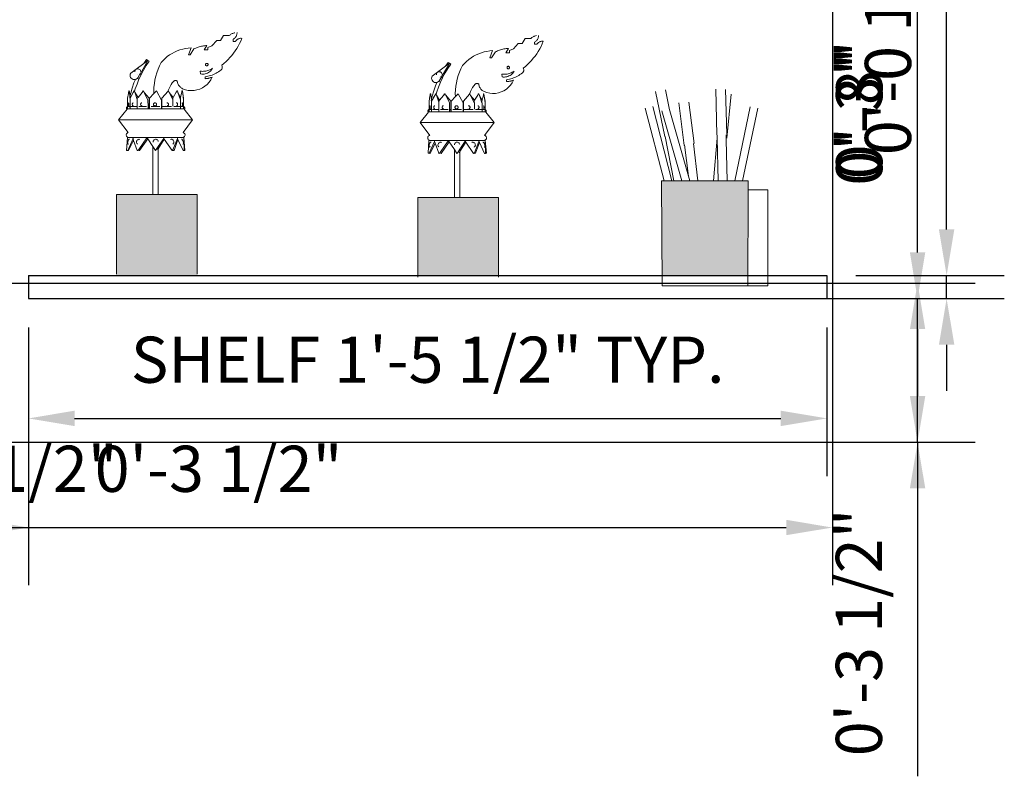
# Model space of a CAD drawing. Units: millimetres. Extents: x 7894 to 8038, y 6851 to 6951.
# Tile 7 of 49: x 7963.22 to 7984.56, y 6854.37 to 6870.77. Entities that reach past the tile are written whole.
import ezdxf

# ---------------------------------------------------------------- set-up
doc = ezdxf.new("R2010")
doc.units = ezdxf.units.MM
for name, color, linetype, lineweight in [('A-ANNO-DIMS', 2, 'Continuous', 18), ('A-FURN-ACCS', 8, 'Continuous', 13), ('A-FURN-SHLF', 7, 'Continuous', 30)]:
    doc.layers.add(name, color=color, linetype=linetype, lineweight=lineweight)
doc.layers.add('A-FURN-ACCS-PATT', color=116, linetype='Continuous', lineweight=9, true_color=0x136734)
doc.styles.get("Standard").update_dxf_attribs({"font": 'arial.ttf'})
doc.dimstyles.new('ISO-25', dxfattribs={"dimtxt": 1, "dimasz": 1, "dimexe": 1.25, "dimexo": 0.625, "dimtad": 1, "dimdec": 0, "dimlunit": 4, "dimtxsty": 'Standard', "dimcen": 2.5, "dimclrt": 1, "dimadec": 0, "dimazin": 0, "dimtfac": 1, "dimtdec": 0, "dimtmove": 0, "dimatfit": 3, "dimfxl": 1, "dimarcsym": 0})

# ---------------------------------------------------------------- blocks, each defined once
blk = doc.blocks.new('FLOATING-SHELF-ELEV')
for p, q in [((0, 0.5), (17.304, 0.5)), ((0, 0.5), (0, 0)), ((17.304, 0.5), (17.304, 0)), ((0, 0), (17.304, 0))]:
    blk.add_line(p, q)
blk = doc.blocks.new('DISPLAY-LEAF-FINIAL')
for p, q in [((2.209, 3.334), (2.276, 3.441)), ((2.276, 3.441), (2.398, 3.441)), ((2.398, 3.441), (2.409, 3.452)), ((2.409, 3.452), (2.421, 3.461)), ((2.421, 3.461), (2.434, 3.47)), ((2.434, 3.47), (2.447, 3.478)), ((2.447, 3.478), (2.461, 3.485)), ((2.461, 3.485), (2.475, 3.491)), ((2.475, 3.491), (2.489, 3.496)), ((2.489, 3.496), (2.504, 3.501)), ((2.504, 3.501), (2.519, 3.504)), ((2.544, 3.424), (2.536, 3.411)), ((2.551, 3.437), (2.544, 3.424)), ((2.556, 3.45), (2.551, 3.437)), ((2.56, 3.465), (2.556, 3.45)), ((2.563, 3.479), (2.56, 3.465)), ((2.565, 3.494), (2.563, 3.479)), ((2.565, 3.508), (2.565, 3.494)), ((1.745, 3.198), (1.769, 3.205)), ((1.769, 3.205), (1.793, 3.211)), ((1.793, 3.211), (1.817, 3.216)), ((1.817, 3.216), (1.841, 3.22)), ((1.841, 3.22), (1.865, 3.223)), ((1.914, 3.227), (1.854, 3.133)), ((1.865, 3.223), (1.889, 3.226)), ((1.889, 3.226), (1.914, 3.227)), ((1.934, 3.185), (2.023, 3.221)), ((2.023, 3.221), (2.127, 3.334)), ((2.127, 3.334), (2.209, 3.334)), ((2.493, 3.371), (2.48, 3.364)), ((2.48, 3.364), (2.48, 3.316)), ((2.48, 3.316), (2.533, 3.316)), ((2.505, 3.379), (2.493, 3.371)), ((2.516, 3.389), (2.505, 3.379)), ((2.527, 3.4), (2.516, 3.389)), ((2.536, 3.411), (2.527, 3.4)), ((2.533, 3.316), (2.54, 3.327)), ((2.54, 3.327), (2.549, 3.338)), ((2.549, 3.338), (2.558, 3.347)), ((2.558, 3.347), (2.569, 3.356)), ((2.591, 3.216), (2.56, 3.163)), ((2.569, 3.356), (2.58, 3.363)), ((2.58, 3.363), (2.592, 3.37)), ((2.62, 3.27), (2.591, 3.216)), ((2.592, 3.37), (2.604, 3.375)), ((2.604, 3.375), (2.617, 3.379)), ((2.617, 3.379), (2.63, 3.382)), ((2.646, 3.325), (2.62, 3.27)), ((2.63, 3.382), (2.643, 3.383)), ((2.643, 3.383), (2.657, 3.383)), ((2.67, 3.382), (2.646, 3.325)), ((2.657, 3.383), (2.67, 3.382)), ((1.055, 2.986), (1.105, 3.023)), ((1.105, 3.023), (1.158, 3.056)), ((1.158, 3.056), (1.213, 3.085)), ((1.213, 3.085), (1.27, 3.111)), ((1.27, 3.111), (1.328, 3.133)), ((1.328, 3.133), (1.388, 3.15)), ((1.388, 3.15), (1.449, 3.164)), ((1.449, 3.164), (1.51, 3.173)), ((1.51, 3.173), (1.572, 3.179)), ((1.572, 3.179), (1.511, 3.024)), ((1.511, 3.024), (1.55, 3.024)), ((1.55, 3.024), (1.632, 3.152)), ((1.632, 3.152), (1.654, 3.163)), ((1.654, 3.163), (1.676, 3.173)), ((1.676, 3.173), (1.699, 3.182)), ((1.699, 3.182), (1.722, 3.191)), ((1.722, 3.191), (1.745, 3.198)), ((1.854, 3.133), (1.934, 3.133)), ((1.934, 3.133), (1.934, 3.185)), ((2.453, 3.014), (2.413, 2.967)), ((2.491, 3.062), (2.453, 3.014)), ((2.527, 3.112), (2.491, 3.062)), ((2.56, 3.163), (2.527, 3.112)), ((0.547, 2.84), (0.379, 2.713)), ((0.634, 2.9), (0.463, 2.609)), ((0.541, 2.696), (0.599, 2.791)), ((0.605, 2.924), (0.547, 2.84)), ((0.634, 2.905), (0.547, 2.84)), ((0.599, 2.791), (0.663, 2.885)), ((0.634, 2.905), (0.605, 2.924)), ((0.634, 2.9), (0.634, 2.905)), ((0.663, 2.885), (0.634, 2.905)), ((0.884, 2.786), (0.853, 2.713)), ((0.92, 2.857), (0.884, 2.786)), ((0.92, 2.857), (0.962, 2.903)), ((0.962, 2.903), (1.007, 2.946)), ((1.007, 2.946), (1.055, 2.986)), ((1.883, 2.817), (1.885, 2.824)), ((1.883, 2.81), (1.883, 2.817)), ((1.885, 2.803), (1.883, 2.81)), ((1.885, 2.824), (1.889, 2.831)), ((1.888, 2.797), (1.885, 2.803)), ((1.894, 2.791), (1.888, 2.797)), ((1.889, 2.831), (1.894, 2.836)), ((1.894, 2.836), (1.9, 2.839)), ((1.9, 2.788), (1.894, 2.791)), ((1.9, 2.839), (1.907, 2.841)), ((1.907, 2.786), (1.9, 2.788)), ((1.907, 2.841), (1.914, 2.841)), ((1.914, 2.786), (1.907, 2.786)), ((1.914, 2.841), (1.921, 2.839)), ((1.921, 2.788), (1.914, 2.786)), ((1.921, 2.839), (1.928, 2.836)), ((1.928, 2.791), (1.921, 2.788)), ((1.928, 2.836), (1.933, 2.83)), ((1.933, 2.796), (1.928, 2.791)), ((1.933, 2.83), (1.937, 2.824)), ((1.936, 2.803), (1.933, 2.796)), ((1.938, 2.81), (1.936, 2.803)), ((1.937, 2.824), (1.938, 2.817)), ((1.938, 2.817), (1.938, 2.81)), ((2.281, 2.839), (2.233, 2.801)), ((2.233, 2.801), (2.238, 2.792)), ((2.238, 2.792), (2.242, 2.783)), ((2.242, 2.783), (2.245, 2.774)), ((2.327, 2.88), (2.281, 2.839)), ((2.371, 2.923), (2.327, 2.88)), ((2.413, 2.967), (2.371, 2.923)), ((0.253, 2.607), (0.249, 2.584)), ((0.249, 2.58), (0.249, 2.584)), ((0.249, 2.58), (0.251, 2.557)), ((0.264, 2.627), (0.253, 2.607)), ((0.379, 2.713), (0.264, 2.627)), ((0.353, 2.675), (0.358, 2.69)), ((0.353, 2.66), (0.353, 2.675)), ((0.353, 2.659), (0.353, 2.66)), ((0.353, 2.657), (0.353, 2.659)), ((0.358, 2.69), (0.367, 2.703)), ((0.367, 2.703), (0.379, 2.713)), ((0.379, 2.713), (0.393, 2.72)), ((0.393, 2.72), (0.409, 2.723)), ((0.409, 2.723), (0.425, 2.722)), ((0.414, 2.606), (0.413, 2.603)), ((0.461, 2.605), (0.415, 2.527)), ((0.425, 2.722), (0.44, 2.718)), ((0.44, 2.718), (0.453, 2.709)), ((0.44, 2.496), (0.486, 2.593)), ((0.443, 2.613), (0.446, 2.612)), ((0.451, 2.615), (0.449, 2.616)), ((0.453, 2.709), (0.464, 2.698)), ((0.463, 2.609), (0.461, 2.605)), ((0.486, 2.593), (0.461, 2.605)), ((0.463, 2.609), (0.488, 2.597)), ((0.464, 2.698), (0.471, 2.684)), ((0.471, 2.684), (0.475, 2.669)), ((0.474, 2.667), (0.475, 2.669)), ((0.474, 2.667), (0.475, 2.666)), ((0.541, 2.696), (0.488, 2.597)), ((0.804, 2.562), (0.787, 2.485)), ((0.826, 2.638), (0.804, 2.562)), ((0.853, 2.713), (0.826, 2.638)), ((1.793, 2.668), (1.77, 2.67)), ((1.77, 2.67), (1.776, 2.611)), ((1.801, 2.608), (1.776, 2.611)), ((1.816, 2.667), (1.793, 2.668)), ((1.827, 2.607), (1.801, 2.608)), ((1.84, 2.668), (1.816, 2.667)), ((1.852, 2.609), (1.827, 2.607)), ((1.863, 2.67), (1.84, 2.668)), ((1.878, 2.613), (1.852, 2.609)), ((1.886, 2.673), (1.863, 2.67)), ((1.902, 2.62), (1.878, 2.613)), ((1.909, 2.678), (1.886, 2.673)), ((1.926, 2.63), (1.902, 2.62)), ((1.931, 2.684), (1.909, 2.678)), ((1.949, 2.642), (1.926, 2.63)), ((1.954, 2.692), (1.931, 2.684)), ((1.964, 2.569), (1.934, 2.561)), ((1.97, 2.657), (1.949, 2.642)), ((1.975, 2.701), (1.954, 2.692)), ((1.994, 2.578), (1.964, 2.569)), ((1.99, 2.673), (1.97, 2.657)), ((1.996, 2.711), (1.975, 2.701)), ((2.007, 2.692), (1.99, 2.673)), ((2.024, 2.588), (1.994, 2.578)), ((2.017, 2.722), (1.996, 2.711)), ((2.023, 2.712), (2.007, 2.692)), ((2.036, 2.734), (2.017, 2.722)), ((2.036, 2.734), (2.023, 2.712)), ((2.053, 2.6), (2.024, 2.588)), ((2.082, 2.613), (2.053, 2.6)), ((2.11, 2.627), (2.082, 2.613)), ((2.137, 2.643), (2.11, 2.627)), ((2.164, 2.659), (2.137, 2.643)), ((2.19, 2.677), (2.164, 2.659)), ((2.216, 2.695), (2.19, 2.677)), ((2.223, 2.702), (2.216, 2.695)), ((2.23, 2.709), (2.223, 2.702)), ((2.235, 2.717), (2.23, 2.709)), ((2.24, 2.726), (2.235, 2.717)), ((2.243, 2.735), (2.24, 2.726)), ((2.245, 2.745), (2.243, 2.735)), ((2.245, 2.774), (2.246, 2.764)), ((2.246, 2.754), (2.245, 2.745)), ((2.246, 2.764), (2.246, 2.754)), ((0.251, 2.557), (0.259, 2.536)), ((0.259, 2.536), (0.272, 2.517)), ((0.272, 2.517), (0.29, 2.502)), ((0.29, 2.502), (0.311, 2.492)), ((0.332, 2.415), (0.295, 2.306)), ((0.311, 2.492), (0.334, 2.488)), ((0.363, 2.491), (0.332, 2.415)), ((0.334, 2.488), (0.358, 2.489)), ((0.358, 2.489), (0.363, 2.491)), ((0.361, 2.285), (0.398, 2.391)), ((0.363, 2.491), (0.38, 2.497)), ((0.365, 2.496), (0.363, 2.491)), ((0.38, 2.497), (0.4, 2.51)), ((0.398, 2.513), (0.402, 2.512)), ((0.398, 2.391), (0.44, 2.495)), ((0.403, 2.513), (0.4, 2.514)), ((0.4, 2.51), (0.402, 2.512)), ((0.402, 2.512), (0.403, 2.513)), ((0.402, 2.512), (0.44, 2.495)), ((0.403, 2.513), (0.415, 2.527)), ((0.403, 2.513), (0.44, 2.496)), ((0.409, 2.511), (0.408, 2.509)), ((0.42, 2.535), (0.409, 2.511)), ((0.774, 2.406), (0.766, 2.327)), ((0.787, 2.485), (0.774, 2.406)), ((1.136, 2.379), (1.113, 2.339)), ((1.163, 2.417), (1.136, 2.379)), ((1.193, 2.452), (1.163, 2.417)), ((1.198, 2.457), (1.193, 2.452)), ((1.204, 2.462), (1.198, 2.457)), ((1.211, 2.465), (1.204, 2.462)), ((1.218, 2.467), (1.211, 2.465)), ((1.225, 2.469), (1.218, 2.467)), ((1.232, 2.47), (1.225, 2.469)), ((1.239, 2.469), (1.232, 2.47)), ((1.247, 2.467), (1.239, 2.469)), ((1.254, 2.465), (1.247, 2.467)), ((1.26, 2.462), (1.254, 2.465)), ((1.266, 2.457), (1.26, 2.462)), ((1.271, 2.452), (1.266, 2.457)), ((1.274, 2.435), (1.271, 2.452)), ((1.278, 2.418), (1.274, 2.435)), ((1.283, 2.402), (1.278, 2.418)), ((1.29, 2.386), (1.283, 2.402)), ((1.298, 2.371), (1.29, 2.386)), ((1.308, 2.357), (1.298, 2.371)), ((1.319, 2.343), (1.308, 2.357)), ((1.918, 2.385), (1.87, 2.344)), ((1.903, 2.554), (1.872, 2.548)), ((1.872, 2.548), (1.872, 2.508)), ((1.872, 2.508), (1.885, 2.509)), ((1.885, 2.509), (1.898, 2.51)), ((1.898, 2.51), (1.911, 2.511)), ((1.934, 2.561), (1.903, 2.554)), ((1.911, 2.511), (1.924, 2.513)), ((1.961, 2.432), (1.918, 2.385)), ((1.924, 2.513), (1.937, 2.515)), ((1.937, 2.515), (1.95, 2.518)), ((1.95, 2.518), (1.963, 2.521)), ((1.997, 2.484), (1.961, 2.432)), ((1.963, 2.521), (1.976, 2.524)), ((1.976, 2.524), (1.988, 2.528)), ((1.988, 2.528), (2.001, 2.532)), ((2.026, 2.541), (1.997, 2.484)), ((2.001, 2.532), (2.013, 2.536)), ((2.013, 2.536), (2.026, 2.541)), ((0.213, 2.19), (0.195, 2.086)), ((0.213, 2.19), (0.215, 2.201)), ((0.215, 2.201), (0.22, 2.245)), ((0.223, 2.245), (0.215, 2.201)), ((0.223, 2.245), (0.22, 2.245)), ((0.223, 2.245), (0.23, 2.245)), ((0.232, 2.22), (0.23, 2.245)), ((0.232, 2.22), (0.25, 2.138)), ((0.244, 2.11), (0.232, 2.22)), ((0.25, 2.138), (0.244, 2.11)), ((0.317, 2.207), (0.248, 2.086)), ((0.263, 2.194), (0.25, 2.138)), ((0.25, 2.138), (0.256, 2.115)), ((0.295, 2.306), (0.263, 2.194)), ((0.297, 2.185), (0.292, 2.162)), ((0.317, 2.207), (0.33, 2.245)), ((0.338, 2.245), (0.317, 2.207)), ((0.332, 2.245), (0.33, 2.245)), ((0.344, 2.245), (0.338, 2.245)), ((0.347, 2.235), (0.344, 2.245)), ((0.347, 2.235), (0.361, 2.285)), ((0.354, 2.213), (0.347, 2.235)), ((0.354, 2.213), (0.42, 2.104)), ((0.404, 2.061), (0.354, 2.213)), ((0.507, 2.209), (0.42, 2.104)), ((0.507, 2.209), (0.525, 2.245)), ((0.532, 2.239), (0.507, 2.209)), ((0.528, 2.245), (0.525, 2.245)), ((0.528, 2.245), (0.532, 2.239)), ((0.537, 2.245), (0.532, 2.239)), ((0.54, 2.245), (0.537, 2.245)), ((0.556, 2.211), (0.54, 2.245)), ((0.548, 2.22), (0.556, 2.211)), ((0.556, 2.211), (0.663, 2.086)), ((0.636, 2.045), (0.556, 2.211)), ((0.765, 2.186), (0.671, 2.086)), ((0.766, 2.327), (0.763, 2.248)), ((0.763, 2.248), (0.765, 2.186)), ((0.821, 2.245), (0.765, 2.186)), ((0.93, 2.045), (0.821, 2.245)), ((1.07, 2.239), (0.939, 2.086)), ((1.07, 2.239), (1.069, 2.235)), ((1.071, 2.24), (1.07, 2.239)), ((1.07, 2.239), (1.071, 2.237)), ((1.075, 2.254), (1.071, 2.24)), ((1.074, 2.245), (1.071, 2.24)), ((1.074, 2.245), (1.078, 2.245)), ((1.092, 2.297), (1.075, 2.254)), ((1.095, 2.209), (1.078, 2.245)), ((1.113, 2.339), (1.092, 2.297)), ((1.095, 2.209), (1.182, 2.104)), ((1.095, 2.209), (1.171, 2.054)), ((1.248, 2.213), (1.182, 2.104)), ((1.248, 2.213), (1.258, 2.245)), ((1.265, 2.242), (1.248, 2.213)), ((1.258, 2.245), (1.264, 2.245)), ((1.264, 2.245), (1.265, 2.242)), ((1.267, 2.245), (1.265, 2.242)), ((1.267, 2.245), (1.272, 2.245)), ((1.285, 2.207), (1.272, 2.245)), ((1.285, 2.207), (1.344, 2.103)), ((1.285, 2.207), (1.34, 2.048)), ((1.331, 2.331), (1.319, 2.343)), ((1.343, 2.319), (1.331, 2.331)), ((1.357, 2.309), (1.343, 2.319)), ((1.37, 2.22), (1.344, 2.103)), ((1.372, 2.3), (1.357, 2.309)), ((1.37, 2.22), (1.372, 2.245)), ((1.375, 2.245), (1.37, 2.22)), ((1.387, 2.292), (1.372, 2.3)), ((1.372, 2.245), (1.375, 2.245)), ((1.375, 2.245), (1.382, 2.245)), ((1.382, 2.245), (1.389, 2.19)), ((1.447, 2.27), (1.387, 2.292)), ((1.389, 2.19), (1.408, 2.086)), ((1.407, 2.045), (1.389, 2.19)), ((1.509, 2.256), (1.447, 2.27)), ((1.572, 2.25), (1.509, 2.256)), ((1.635, 2.253), (1.572, 2.25)), ((1.698, 2.264), (1.635, 2.253)), ((1.759, 2.283), (1.698, 2.264)), ((1.816, 2.31), (1.759, 2.283)), ((1.87, 2.344), (1.816, 2.31)), ((0.195, 2.086), (0.195, 2.048)), ((0.195, 2.045), (0.195, 2.048)), ((0.195, 2.045), (0.195, 1.903)), ((0.207, 1.965), (0.208, 1.973)), ((0.207, 1.956), (0.207, 1.965)), ((0.207, 1.947), (0.207, 1.956)), ((0.207, 1.938), (0.207, 1.947)), ((0.208, 1.93), (0.207, 1.938)), ((0.208, 1.973), (0.209, 1.979)), ((0.209, 1.924), (0.208, 1.93)), ((0.209, 1.979), (0.211, 1.984)), ((0.211, 1.919), (0.209, 1.924)), ((0.21, 1.956), (0.211, 1.965)), ((0.21, 1.947), (0.21, 1.956)), ((0.211, 1.938), (0.21, 1.947)), ((0.211, 1.984), (0.213, 1.986)), ((0.211, 1.965), (0.212, 1.973)), ((0.212, 1.93), (0.211, 1.938)), ((0.212, 1.973), (0.213, 1.979)), ((0.213, 1.924), (0.212, 1.93)), ((0.216, 1.986), (0.213, 1.986)), ((0.213, 1.979), (0.214, 1.984)), ((0.216, 1.947), (0.213, 1.924)), ((0.214, 1.919), (0.213, 1.924)), ((0.214, 1.984), (0.216, 1.986)), ((0.217, 1.965), (0.216, 1.956)), ((0.216, 1.956), (0.216, 1.947)), ((0.216, 1.947), (0.217, 1.938)), ((0.218, 1.973), (0.217, 1.965)), ((0.218, 1.967), (0.217, 1.965)), ((0.217, 1.938), (0.218, 1.93)), ((0.219, 1.979), (0.218, 1.973)), ((0.218, 1.973), (0.218, 1.967)), ((0.218, 1.93), (0.219, 1.924)), ((0.22, 1.981), (0.219, 1.979)), ((0.22, 1.981), (0.219, 1.979)), ((0.219, 1.924), (0.22, 1.921)), ((0.221, 1.973), (0.22, 1.965)), ((0.22, 1.965), (0.22, 1.956)), ((0.22, 1.956), (0.22, 1.947)), ((0.22, 1.947), (0.22, 1.938)), ((0.22, 1.938), (0.221, 1.93)), ((0.222, 1.975), (0.221, 1.973)), ((0.221, 1.93), (0.222, 1.928)), ((0.244, 2.11), (0.239, 2.089)), ((0.248, 2.065), (0.244, 2.11)), ((0.248, 1.925), (0.246, 1.901)), ((0.248, 2.086), (0.248, 2.065)), ((0.248, 2.065), (0.248, 1.903)), ((0.295, 1.956), (0.297, 1.965)), ((0.295, 1.947), (0.295, 1.956)), ((0.297, 1.938), (0.295, 1.947)), ((0.297, 1.965), (0.3, 1.973)), ((0.3, 1.93), (0.297, 1.938)), ((0.3, 1.973), (0.304, 1.979)), ((0.303, 1.924), (0.3, 1.93)), ((0.308, 1.919), (0.303, 1.924)), ((0.304, 1.979), (0.308, 1.984)), ((0.308, 1.984), (0.314, 1.986)), ((0.316, 1.986), (0.314, 1.986)), ((0.42, 2.104), (0.404, 2.086)), ((0.404, 2.086), (0.404, 2.061)), ((0.404, 2.061), (0.404, 1.901)), ((0.476, 1.956), (0.478, 1.965)), ((0.476, 1.947), (0.476, 1.956)), ((0.478, 1.938), (0.476, 1.947)), ((0.478, 1.965), (0.482, 1.973)), ((0.482, 1.93), (0.478, 1.938)), ((0.482, 1.973), (0.488, 1.979)), ((0.488, 1.924), (0.482, 1.93)), ((0.488, 1.979), (0.495, 1.984)), ((0.495, 1.919), (0.488, 1.924)), ((0.495, 1.984), (0.502, 1.986)), ((0.504, 1.986), (0.502, 1.986)), ((0.636, 2.045), (0.637, 1.903)), ((0.663, 2.086), (0.663, 1.903)), ((0.671, 2.086), (0.671, 1.903)), ((0.754, 1.956), (0.756, 1.965)), ((0.754, 1.947), (0.754, 1.956)), ((0.756, 1.938), (0.754, 1.947)), ((0.756, 1.965), (0.761, 1.973)), ((0.761, 1.93), (0.756, 1.938)), ((0.761, 1.973), (0.767, 1.979)), ((0.767, 1.924), (0.761, 1.93)), ((0.767, 1.979), (0.775, 1.984)), ((0.775, 1.919), (0.767, 1.924)), ((0.775, 1.984), (0.784, 1.986)), ((0.784, 1.986), (0.793, 1.986)), ((0.793, 1.986), (0.802, 1.984)), ((0.802, 1.984), (0.81, 1.979)), ((0.81, 1.924), (0.802, 1.919)), ((0.81, 1.979), (0.816, 1.973)), ((0.816, 1.93), (0.81, 1.924)), ((0.816, 1.973), (0.821, 1.965)), ((0.821, 1.938), (0.816, 1.93)), ((0.821, 1.965), (0.823, 1.956)), ((0.823, 1.947), (0.821, 1.938)), ((0.823, 1.956), (0.823, 1.947)), ((0.93, 2.045), (0.931, 1.934)), ((0.939, 1.934), (0.931, 1.934)), ((0.931, 1.934), (0.931, 1.903)), ((0.939, 2.086), (0.939, 1.934)), ((0.942, 1.934), (0.939, 1.934)), ((0.939, 1.934), (0.939, 1.903)), ((1.022, 1.935), (1.021, 1.935)), ((1.044, 1.986), (1.046, 1.986)), ((1.046, 1.986), (1.054, 1.986)), ((1.054, 1.986), (1.062, 1.984)), ((1.062, 1.984), (1.069, 1.979)), ((1.069, 1.924), (1.062, 1.919)), ((1.069, 1.979), (1.075, 1.973)), ((1.075, 1.93), (1.069, 1.924)), ((1.075, 1.973), (1.079, 1.965)), ((1.079, 1.938), (1.075, 1.93)), ((1.079, 1.965), (1.081, 1.956)), ((1.081, 1.947), (1.079, 1.938)), ((1.081, 1.956), (1.081, 1.947)), ((1.182, 2.104), (1.171, 2.086)), ((1.171, 2.086), (1.171, 2.054)), ((1.176, 2.045), (1.171, 2.054)), ((1.176, 2.045), (1.177, 1.914)), ((1.249, 1.986), (1.251, 1.986)), ((1.251, 1.986), (1.257, 1.986)), ((1.257, 1.986), (1.263, 1.984)), ((1.263, 1.984), (1.268, 1.979)), ((1.268, 1.924), (1.263, 1.919)), ((1.268, 1.979), (1.272, 1.973)), ((1.272, 1.93), (1.268, 1.924)), ((1.272, 1.973), (1.275, 1.965)), ((1.275, 1.938), (1.272, 1.93)), ((1.275, 1.965), (1.276, 1.956)), ((1.276, 1.947), (1.275, 1.938)), ((1.276, 1.956), (1.276, 1.947)), ((1.344, 2.103), (1.34, 2.086)), ((1.34, 2.086), (1.34, 2.048)), ((1.341, 2.045), (1.34, 2.048)), ((1.341, 2.045), (1.342, 1.903)), ((1.373, 1.986), (1.376, 1.986)), ((1.376, 1.986), (1.378, 1.984)), ((1.376, 1.986), (1.377, 1.986)), ((1.377, 1.986), (1.379, 1.986)), ((1.378, 1.984), (1.379, 1.979)), ((1.379, 1.924), (1.378, 1.919)), ((1.379, 1.986), (1.381, 1.984)), ((1.379, 1.979), (1.381, 1.973)), ((1.381, 1.93), (1.379, 1.924)), ((1.381, 1.984), (1.383, 1.979)), ((1.381, 1.973), (1.382, 1.965)), ((1.382, 1.938), (1.381, 1.93)), ((1.383, 1.924), (1.381, 1.919)), ((1.382, 1.965), (1.382, 1.956)), ((1.382, 1.956), (1.382, 1.947)), ((1.382, 1.947), (1.382, 1.938)), ((1.383, 1.979), (1.384, 1.973)), ((1.384, 1.93), (1.383, 1.924)), ((1.384, 1.973), (1.385, 1.965)), ((1.385, 1.938), (1.384, 1.93)), ((1.385, 1.965), (1.386, 1.956)), ((1.386, 1.947), (1.385, 1.938)), ((1.386, 1.956), (1.386, 1.947)), ((1.408, 2.086), (1.407, 2.045)), ((1.407, 2.045), (1.408, 1.903)), ((0, 1.62), (0.181, 1.849)), ((0.17, 1.877), (0.172, 1.885)), ((0.17, 1.87), (0.17, 1.877)), ((0.172, 1.862), (0.17, 1.87)), ((0.172, 1.885), (0.176, 1.892)), ((0.175, 1.855), (0.172, 1.862)), ((0.181, 1.849), (0.175, 1.855)), ((0.176, 1.892), (0.182, 1.898)), ((0.182, 1.898), (0.189, 1.901)), ((0.189, 1.901), (0.195, 1.903)), ((0.195, 1.903), (0.195, 1.901)), ((0.195, 1.903), (0.196, 1.903)), ((0.195, 1.898), (0.195, 1.87)), ((0.195, 1.862), (0.195, 1.855)), ((0.195, 1.855), (0.195, 1.855)), ((0.205, 1.855), (0.195, 1.855)), ((0.196, 1.903), (0.198, 1.903)), ((0.196, 1.903), (0.197, 1.903)), ((0.237, 1.903), (0.198, 1.903)), ((0.205, 1.855), (0.205, 1.851)), ((0.248, 1.855), (0.205, 1.855)), ((0.205, 1.851), (0.205, 1.849)), ((0.213, 1.917), (0.211, 1.919)), ((0.214, 1.917), (0.213, 1.917)), ((0.216, 1.917), (0.214, 1.919)), ((0.216, 1.917), (0.214, 1.917)), ((0.218, 1.917), (0.216, 1.917)), ((0.24, 1.855), (0.24, 1.849)), ((0.248, 1.903), (0.244, 1.903)), ((0.245, 1.898), (0.244, 1.886)), ((0.248, 1.897), (0.244, 1.897)), ((0.248, 1.903), (0.248, 1.901)), ((0.248, 1.898), (0.248, 1.897)), ((0.248, 1.897), (0.248, 1.87)), ((0.248, 1.862), (0.248, 1.855)), ((0.248, 1.855), (0.276, 1.855)), ((0.391, 1.903), (0.265, 1.903)), ((0.275, 1.849), (0.276, 1.855)), ((0.276, 1.855), (0.405, 1.855)), ((0.313, 1.917), (0.308, 1.919)), ((0.319, 1.917), (0.313, 1.917)), ((0.322, 1.917), (0.319, 1.917)), ((0.404, 1.898), (0.404, 1.87)), ((0.404, 1.862), (0.405, 1.855)), ((0.405, 1.855), (0.637, 1.855)), ((0.439, 1.903), (0.607, 1.903)), ((0.502, 1.917), (0.495, 1.919)), ((0.51, 1.917), (0.502, 1.917)), ((0.512, 1.917), (0.51, 1.917)), ((0.637, 1.903), (0.634, 1.903)), ((0.637, 1.897), (0.634, 1.897)), ((0.637, 1.903), (0.637, 1.901)), ((0.663, 1.903), (0.637, 1.903)), ((0.637, 1.898), (0.637, 1.897)), ((0.637, 1.897), (0.637, 1.87)), ((0.663, 1.897), (0.637, 1.897)), ((0.637, 1.862), (0.637, 1.855)), ((0.663, 1.855), (0.637, 1.855)), ((0.663, 1.903), (0.671, 1.903)), ((0.663, 1.903), (0.663, 1.901)), ((0.663, 1.898), (0.663, 1.897)), ((0.663, 1.897), (0.663, 1.87)), ((0.671, 1.897), (0.663, 1.897)), ((0.663, 1.862), (0.663, 1.855)), ((0.671, 1.903), (0.671, 1.901)), ((0.671, 1.898), (0.671, 1.897)), ((0.671, 1.897), (0.671, 1.87)), ((0.671, 1.862), (0.671, 1.855)), ((0.671, 1.855), (0.932, 1.855)), ((0.708, 1.903), (0.894, 1.903)), ((0.784, 1.917), (0.775, 1.919)), ((0.793, 1.917), (0.784, 1.917)), ((0.802, 1.919), (0.793, 1.917)), ((0.931, 1.903), (0.931, 1.901)), ((0.939, 1.903), (0.931, 1.903)), ((0.931, 1.898), (0.931, 1.897)), ((0.931, 1.897), (0.932, 1.87)), ((0.939, 1.897), (0.931, 1.897)), ((0.932, 1.862), (0.932, 1.855)), ((0.939, 1.855), (0.932, 1.855)), ((0.942, 1.903), (0.939, 1.903)), ((0.939, 1.903), (0.939, 1.901)), ((0.939, 1.898), (0.939, 1.897)), ((0.942, 1.897), (0.939, 1.897)), ((0.939, 1.897), (0.939, 1.87)), ((0.939, 1.862), (0.939, 1.855)), ((1.342, 1.855), (0.939, 1.855)), ((0.953, 1.903), (1.146, 1.903)), ((1.052, 1.917), (1.054, 1.917)), ((1.062, 1.919), (1.054, 1.917)), ((1.33, 1.903), (1.197, 1.903)), ((1.254, 1.917), (1.257, 1.917)), ((1.263, 1.919), (1.257, 1.917)), ((1.347, 1.903), (1.342, 1.903)), ((1.342, 1.903), (1.342, 1.901)), ((1.342, 1.898), (1.342, 1.897)), ((1.347, 1.897), (1.342, 1.897)), ((1.342, 1.897), (1.342, 1.87)), ((1.342, 1.862), (1.342, 1.855)), ((1.408, 1.855), (1.342, 1.855)), ((1.356, 1.903), (1.4, 1.903)), ((1.378, 1.919), (1.375, 1.917)), ((1.375, 1.917), (1.379, 1.917)), ((1.381, 1.919), (1.379, 1.917)), ((1.408, 1.903), (1.413, 1.901)), ((1.408, 1.903), (1.408, 1.901)), ((1.408, 1.898), (1.408, 1.87)), ((1.408, 1.862), (1.408, 1.855)), ((1.413, 1.901), (1.42, 1.898)), ((1.42, 1.898), (1.426, 1.892)), ((1.427, 1.855), (1.421, 1.849)), ((1.421, 1.849), (1.602, 1.62)), ((1.426, 1.892), (1.43, 1.885)), ((1.431, 1.862), (1.427, 1.855)), ((1.43, 1.885), (1.432, 1.877)), ((1.433, 1.87), (1.431, 1.862)), ((1.432, 1.877), (1.433, 1.87)), ((0.207, 1.343), (0, 1.62)), ((1.602, 1.62), (0, 1.62)), ((1.602, 1.62), (1.395, 1.343)), ((0.164, 1.297), (0.168, 1.31)), ((0.164, 1.283), (0.164, 1.297)), ((0.167, 1.27), (0.164, 1.283)), ((0.168, 1.31), (0.174, 1.321)), ((0.174, 1.321), (0.183, 1.331)), ((0.183, 1.331), (0.195, 1.338)), ((0.195, 1.338), (0.207, 1.343)), ((1.395, 1.343), (1.408, 1.338)), ((1.408, 1.338), (1.419, 1.331)), ((1.419, 1.331), (1.428, 1.321)), ((1.428, 1.321), (1.434, 1.31)), ((1.434, 1.31), (1.438, 1.297)), ((1.438, 1.283), (1.435, 1.27)), ((1.438, 1.297), (1.438, 1.283)), ((0.173, 1.258), (0.167, 1.27)), ((0.171, 0.955), (0.191, 1.234)), ((0.182, 1.248), (0.173, 1.258)), ((0.193, 1.24), (0.182, 1.248)), ((0.219, 1.234), (0.191, 1.234)), ((0.206, 1.236), (0.193, 1.24)), ((0.194, 1.111), (0.196, 1.124)), ((0.195, 1.101), (0.194, 1.111)), ((0.196, 1.094), (0.195, 1.101)), ((0.196, 0.954), (0.311, 1.21)), ((0.196, 1.124), (0.198, 1.137)), ((0.199, 1.09), (0.196, 1.094)), ((0.198, 1.137), (0.202, 1.152)), ((0.203, 1.089), (0.199, 1.09)), ((0.202, 1.152), (0.206, 1.165)), ((0.204, 1.088), (0.203, 1.089)), ((0.219, 1.234), (0.206, 1.236)), ((0.206, 1.165), (0.212, 1.177)), ((0.211, 1.096), (0.213, 1.092)), ((0.212, 1.177), (0.217, 1.187)), ((0.213, 1.092), (0.214, 1.092)), ((0.214, 1.1), (0.214, 1.098)), ((0.215, 0.949), (0.324, 1.172)), ((0.217, 1.187), (0.223, 1.193)), ((0.219, 1.234), (0.297, 1.234)), ((0.223, 1.193), (0.228, 1.197)), ((0.228, 1.197), (0.232, 1.196)), ((0.232, 1.195), (0.232, 1.196)), ((0.232, 1.195), (0.237, 1.195)), ((0.297, 1.234), (0.302, 1.234)), ((0.303, 1.232), (0.297, 1.234)), ((0.303, 1.232), (0.302, 1.234)), ((0.302, 1.234), (0.594, 1.234)), ((0.311, 1.21), (0.303, 1.232)), ((0.324, 1.172), (0.311, 1.21)), ((0.402, 0.955), (0.324, 1.172)), ((0.387, 1.137), (0.389, 1.152)), ((0.387, 1.124), (0.387, 1.137)), ((0.391, 1.111), (0.387, 1.124)), ((0.389, 1.152), (0.395, 1.165)), ((0.397, 1.101), (0.391, 1.111)), ((0.395, 1.165), (0.403, 1.177)), ((0.406, 1.094), (0.397, 1.101)), ((0.403, 1.177), (0.413, 1.187)), ((0.409, 1.092), (0.406, 1.094)), ((0.413, 1.187), (0.424, 1.193)), ((0.424, 1.193), (0.436, 1.197)), ((0.434, 0.975), (0.609, 1.228)), ((0.436, 1.197), (0.448, 1.196)), ((0.448, 1.196), (0.458, 1.192)), ((0.455, 0.949), (0.632, 1.205)), ((0.458, 1.192), (0.461, 1.191)), ((0.594, 1.234), (0.617, 1.234)), ((0.609, 1.228), (0.594, 1.234)), ((0.617, 1.228), (0.617, 1.234)), ((0.952, 1.234), (0.617, 1.234)), ((0.632, 1.205), (0.617, 1.228)), ((0.742, 1.037), (0.632, 1.205)), ((0.747, 1.137), (0.748, 1.152)), ((0.747, 1.136), (0.747, 1.137)), ((0.748, 1.152), (0.752, 1.165)), ((0.752, 1.165), (0.76, 1.177)), ((0.76, 1.177), (0.77, 1.187)), ((0.77, 1.187), (0.783, 1.193)), ((0.783, 1.193), (0.797, 1.197)), ((0.797, 1.197), (0.812, 1.196)), ((0.812, 1.196), (0.826, 1.192)), ((0.826, 1.192), (0.838, 1.185)), ((0.838, 1.185), (0.848, 1.175)), ((0.848, 1.175), (0.855, 1.162)), ((0.855, 1.162), (0.859, 1.148)), ((0.859, 1.147), (0.859, 1.148)), ((0.86, 1.041), (0.977, 1.215)), ((0.86, 0.992), (0.99, 1.195)), ((0.981, 1.234), (0.952, 1.234)), ((0.977, 1.215), (0.974, 1.218)), ((0.99, 1.195), (0.977, 1.215)), ((0.981, 1.234), (0.982, 1.234)), ((0.982, 1.234), (0.983, 1.234)), ((1.284, 1.234), (0.983, 1.234)), ((1.16, 0.949), (0.99, 1.195)), ((1.124, 1.192), (1.126, 1.193)), ((1.126, 1.193), (1.127, 1.193)), ((1.127, 1.193), (1.138, 1.197)), ((1.138, 1.197), (1.15, 1.196)), ((1.15, 1.196), (1.162, 1.192)), ((1.162, 1.192), (1.174, 1.185)), ((1.174, 1.092), (1.172, 1.091)), ((1.174, 1.185), (1.184, 1.175)), ((1.174, 1.092), (1.175, 1.092)), ((1.185, 1.099), (1.175, 1.092)), ((1.177, 0.964), (1.275, 1.212)), ((1.184, 1.175), (1.191, 1.162)), ((1.192, 1.109), (1.185, 1.099)), ((1.191, 1.162), (1.196, 1.148)), ((1.196, 1.121), (1.192, 1.109)), ((1.196, 1.148), (1.198, 1.134)), ((1.198, 1.134), (1.196, 1.121)), ((1.202, 0.955), (1.285, 1.19)), ((1.275, 1.212), (1.283, 1.232)), ((1.285, 1.19), (1.275, 1.212)), ((1.283, 1.232), (1.29, 1.234)), ((1.283, 1.232), (1.284, 1.234)), ((1.284, 1.234), (1.29, 1.234)), ((1.398, 0.949), (1.285, 1.19)), ((1.29, 1.234), (1.383, 1.234)), ((1.359, 1.195), (1.364, 1.197)), ((1.359, 1.195), (1.362, 1.195)), ((1.364, 1.197), (1.369, 1.196)), ((1.369, 1.196), (1.374, 1.192)), ((1.374, 1.192), (1.38, 1.185)), ((1.38, 1.185), (1.386, 1.175)), ((1.397, 1.236), (1.383, 1.234)), ((1.41, 1.234), (1.383, 1.234)), ((1.386, 1.175), (1.392, 1.162)), ((1.392, 1.089), (1.39, 1.088)), ((1.39, 1.088), (1.395, 1.089)), ((1.392, 1.162), (1.396, 1.148)), ((1.399, 1.092), (1.395, 1.089)), ((1.396, 1.148), (1.4, 1.134)), ((1.409, 1.24), (1.397, 1.236)), ((1.401, 1.099), (1.399, 1.092)), ((1.4, 1.134), (1.402, 1.121)), ((1.402, 1.109), (1.401, 1.099)), ((1.402, 1.121), (1.402, 1.109)), ((1.42, 1.248), (1.409, 1.24)), ((1.411, 1.234), (1.41, 1.234)), ((1.411, 1.232), (1.411, 1.234)), ((1.435, 0.955), (1.411, 1.232)), ((1.42, 0.955), (1.411, 1.232)), ((1.429, 1.258), (1.42, 1.248)), ((1.435, 1.27), (1.429, 1.258)), ((0.194, 0.949), (0.171, 0.955)), ((0.194, 0.949), (0.196, 0.954)), ((0.215, 0.949), (0.196, 0.954)), ((0.416, 0.949), (0.402, 0.955)), ((0.416, 0.949), (0.434, 0.975)), ((0.442, 0.955), (0.434, 0.975)), ((0.455, 0.949), (0.442, 0.955)), ((0.742, 0), (0.742, 1.037)), ((0.799, 0.949), (0.742, 1.037)), ((0.799, 0.949), (0.816, 0.974)), ((0.816, 0.974), (0.814, 0.977)), ((0.816, 0.974), (0.86, 1.041)), ((0.816, 0.973), (0.816, 0.974)), ((0.843, 0.965), (0.86, 0.992)), ((0.86, 1.041), (0.86, 1.047)), ((0.86, 0.992), (0.86, 1.041)), ((0.86, 0), (0.86, 0.992)), ((1.16, 0.949), (1.173, 0.955)), ((1.173, 0.955), (1.177, 0.964)), ((1.187, 0.949), (1.177, 0.964)), ((1.187, 0.949), (1.202, 0.955)), ((1.398, 0.949), (1.41, 0.953)), ((1.41, 0.953), (1.42, 0.955)), ((1.412, 0.949), (1.41, 0.953)), ((1.412, 0.949), (1.435, 0.955))]:
    blk.add_line(p, q)
blk = doc.blocks.new('DISPLAY-REED-SPRAY')
for p, q in [((0.218, 1.934), (0.42, 0.963)), ((0.515, 1.573), (0.435, 1.972)), ((1.548, 0.994), (1.529, 1.989)), ((1.766, 1.01), (1.742, 1.98)), ((1.77, 0.926), (1.861, 1.878)), ((0, 1.572), (0.406, 0.001)), ((0.578, 0.003), (0.162, 1.611)), ((0.792, 0), (0.361, 1.519)), ((0.935, 0.103), (0.519, 1.567)), ((0.846, 0.767), (0.729, 1.689)), ((1.062, 0.811), (0.945, 1.707)), ((1.938, 0.003), (2.275, 1.603)), ((2.108, 0.001), (2.44, 1.573)), ((0.62, 0.003), (0.428, 0.96)), ((1.477, 0.003), (1.56, 0.927)), ((1.56, 0.991), (1.561, 0.935)), ((1.56, 0.927), (1.561, 0.935)), ((1.56, 0.927), (1.58, 0.003)), ((1.753, 0.892), (1.751, 0.999)), ((1.753, 0.892), (1.755, 0.914)), ((1.771, 0.003), (1.753, 0.892)), ((0.935, 0.103), (0.852, 0.78)), ((1.139, 0.003), (1.042, 0.808)), ((0.963, 0.002), (0.935, 0.103))]:
    blk.add_line(p, q)
blk = doc.blocks.new('*D21')
at = {"layer": 'A-ANNO-DIMS', "color": 0, "lineweight": -2, "transparency": 16777216}
for p, q in [((7963.414, 6864.097), (7963.414, 6860.877)), ((7980.718, 6864.097), (7980.718, 6860.877)), ((7964.414, 6862.127), (7979.718, 6862.127))]:
    blk.add_line(p, q, dxfattribs=at)
at = {"layer": 'A-ANNO-DIMS', "color": 0, "transparency": 16777216}
for points in [[(7964.414, 6862.294), (7964.414, 6861.96), (7963.414, 6862.127)], [(7979.718, 6862.294), (7979.718, 6861.96), (7980.718, 6862.127)]]:
    blk.add_solid(points, dxfattribs=at)
at = {"layer": 'Defpoints', "color": 0, "transparency": 16777216}
for p in [(7963.414, 6864.722), (7980.718, 6864.722), (7980.718, 6862.127)]:
    blk.add_point(p, dxfattribs=at)
at = {"layer": 'A-ANNO-DIMS', "color": 1, "transparency": 16777216, "insert": (7972.066, 6863.269), "char_height": 1, "attachment_point": 5}
blk.add_mtext('SHELF 1\'-5 1/2" TYP.', dxfattribs=at)
blk = doc.blocks.new('*D22')
at = {"layer": 'A-ANNO-DIMS', "color": 0, "lineweight": -2, "transparency": 16777216}
for p, q in [((7983.313, 6866.222), (7983.313, 6876.898)), ((7981.343, 6865.222), (7984.563, 6865.222)), ((7983.313, 6864.722), (7983.313, 6865.222)), ((7981.343, 6864.722), (7984.563, 6864.722)), ((7983.313, 6863.722), (7983.313, 6862.722))]:
    blk.add_line(p, q, dxfattribs=at)
at = {"layer": 'A-ANNO-DIMS', "color": 0, "transparency": 16777216}
for points in [[(7983.146, 6866.222), (7983.48, 6866.222), (7983.313, 6865.222)], [(7983.146, 6863.722), (7983.48, 6863.722), (7983.313, 6864.722)]]:
    blk.add_solid(points, dxfattribs=at)
at = {"layer": 'Defpoints', "color": 0, "transparency": 16777216}
for p in [(7980.718, 6865.222), (7983.313, 6865.222), (7980.718, 6864.722)]:
    blk.add_point(p, dxfattribs=at)
at = {"layer": 'A-ANNO-DIMS', "color": 1, "transparency": 16777216, "insert": (7982.171, 6872.06), "char_height": 1, "attachment_point": 5, "rotation": 90}
blk.add_mtext('0\'-0 1/2" TYP.', dxfattribs=at)
blk = doc.blocks.new('*D36')
at = {"layer": 'A-ANNO-DIMS', "color": 0, "lineweight": -2, "transparency": 16777216}
for p, q in [((7980.836, 6877.959), (7980.836, 6858.512)), ((7944.487, 6864.436), (7944.487, 6858.512)), ((7945.487, 6859.762), (7979.836, 6859.762))]:
    blk.add_line(p, q, dxfattribs=at)
at = {"layer": 'A-ANNO-DIMS', "color": 0, "transparency": 16777216}
for points in [[(7945.487, 6859.929), (7945.487, 6859.596), (7944.487, 6859.762)], [(7979.836, 6859.929), (7979.836, 6859.596), (7980.836, 6859.762)]]:
    blk.add_solid(points, dxfattribs=at)
at = {"layer": 'Defpoints', "color": 0, "transparency": 16777216}
for p in [(7980.836, 6878.584), (7944.487, 6865.061), (7980.836, 6859.762)]:
    blk.add_point(p, dxfattribs=at)
at = {"layer": 'A-ANNO-DIMS', "color": 1, "transparency": 16777216, "insert": (7962.661, 6860.905), "char_height": 1, "attachment_point": 5}
blk.add_mtext('3\'-0 1/2"', dxfattribs=at)
blk = doc.blocks.new('*D38')
at = {"layer": 'A-ANNO-DIMS', "color": 0, "lineweight": -2, "transparency": 16777216}
for p, q in [((7981.461, 6872.903), (7983.933, 6872.903)), ((7982.683, 6865.722), (7982.683, 6871.903)), ((7981.343, 6864.722), (7983.933, 6864.722))]:
    blk.add_line(p, q, dxfattribs=at)
at = {"layer": 'A-ANNO-DIMS', "color": 0, "transparency": 16777216}
for points in [[(7982.517, 6871.903), (7982.85, 6871.903), (7982.683, 6872.903)], [(7982.517, 6865.722), (7982.85, 6865.722), (7982.683, 6864.722)]]:
    blk.add_solid(points, dxfattribs=at)
at = {"layer": 'Defpoints', "color": 0, "transparency": 16777216}
for p in [(7980.836, 6872.903), (7982.683, 6872.903), (7980.718, 6864.722)]:
    blk.add_point(p, dxfattribs=at)
at = {"layer": 'A-ANNO-DIMS', "color": 1, "transparency": 16777216, "insert": (7981.548, 6868.813), "char_height": 1, "attachment_point": 5, "rotation": 90}
blk.add_mtext('0\'-8"', dxfattribs=at)
blk = doc.blocks.new('*D41')
at = {"layer": 'A-ANNO-DIMS', "color": 0, "lineweight": -2, "transparency": 16777216}
for p, q in [((7982.683, 6865.722), (7982.683, 6870.631)), ((7964.039, 6864.722), (7983.933, 6864.722)), ((7982.683, 6861.61), (7982.683, 6864.722)), ((7960.773, 6861.61), (7983.933, 6861.61)), ((7982.683, 6860.61), (7982.683, 6859.61))]:
    blk.add_line(p, q, dxfattribs=at)
at = {"layer": 'A-ANNO-DIMS', "color": 0, "transparency": 16777216}
for points in [[(7982.517, 6865.722), (7982.85, 6865.722), (7982.683, 6864.722)], [(7982.517, 6860.61), (7982.85, 6860.61), (7982.683, 6861.61)]]:
    blk.add_solid(points, dxfattribs=at)
at = {"layer": 'Defpoints', "color": 0, "transparency": 16777216}
for p in [(7963.414, 6864.722), (7982.683, 6864.722), (7960.148, 6861.61)]:
    blk.add_point(p, dxfattribs=at)
at = {"layer": 'A-ANNO-DIMS', "color": 1, "transparency": 16777216, "insert": (7981.548, 6868.677), "char_height": 1, "attachment_point": 5, "rotation": 90}
blk.add_mtext('0\'-3"', dxfattribs=at)
blk = doc.blocks.new('*D44')
at = {"layer": 'A-ANNO-DIMS', "color": 0, "lineweight": -2, "transparency": 16777216}
for p, q in [((7963.414, 6864.097), (7963.414, 6858.512)), ((7960.148, 6860.985), (7960.148, 6858.512)), ((7961.148, 6859.762), (7962.414, 6859.762)), ((7963.414, 6859.762), (7970.652, 6859.762))]:
    blk.add_line(p, q, dxfattribs=at)
at = {"layer": 'A-ANNO-DIMS', "color": 0, "transparency": 16777216}
for points in [[(7961.148, 6859.929), (7961.148, 6859.596), (7960.148, 6859.762)], [(7962.414, 6859.929), (7962.414, 6859.596), (7963.414, 6859.762)]]:
    blk.add_solid(points, dxfattribs=at)
at = {"layer": 'Defpoints', "color": 0, "transparency": 16777216}
for p in [(7963.414, 6864.722), (7960.148, 6861.61), (7963.414, 6859.762)]:
    blk.add_point(p, dxfattribs=at)
at = {"layer": 'A-ANNO-DIMS', "color": 1, "transparency": 16777216, "insert": (7967.533, 6860.905), "char_height": 1, "attachment_point": 5}
blk.add_mtext('0\'-3 1/2"', dxfattribs=at)
blk = doc.blocks.new('*D45')
at = {"layer": 'A-ANNO-DIMS', "color": 0, "lineweight": -2, "transparency": 16777216}
for p, q in [((7956.512, 6865.061), (7983.933, 6865.061)), ((7982.683, 6864.061), (7982.683, 6862.61)), ((7960.773, 6861.61), (7983.933, 6861.61)), ((7982.683, 6861.61), (7982.683, 6854.371))]:
    blk.add_line(p, q, dxfattribs=at)
at = {"layer": 'A-ANNO-DIMS', "color": 0, "transparency": 16777216}
for points in [[(7982.517, 6864.061), (7982.85, 6864.061), (7982.683, 6865.061)], [(7982.517, 6862.61), (7982.85, 6862.61), (7982.683, 6861.61)]]:
    blk.add_solid(points, dxfattribs=at)
at = {"layer": 'Defpoints', "color": 0, "transparency": 16777216}
for p in [(7955.887, 6865.061), (7960.148, 6861.61), (7982.683, 6861.61)]:
    blk.add_point(p, dxfattribs=at)
at = {"layer": 'A-ANNO-DIMS', "color": 1, "transparency": 16777216, "insert": (7981.541, 6857.49), "char_height": 1, "attachment_point": 5, "rotation": 90}
blk.add_mtext('0\'-3 1/2"', dxfattribs=at)

msp = doc.modelspace()

# ---------------------------------------------------------------- hatches: boundary and pattern name
at = {"layer": 'A-FURN-ACCS-PATT'}
h = msp.add_hatch(color=256, dxfattribs=at)
h.dxf.hatch_style = 1
h.paths.add_polyline_path([(7966.481, 6880.843), (7965.643, 6880.843), (7965.524, 6880.843), (7964.733, 6880.843), (7964.733, 6879.084), (7966.481, 6879.084)])
h.paths.add_polyline_path([(7967.067, 6866.98), (7966.229, 6866.98), (7966.11, 6866.98), (7965.32, 6866.98), (7965.32, 6865.222), (7967.067, 6865.222)])
h.paths.add_polyline_path([(7979.013, 6867.08), (7979.013, 6867.278), (7978.976, 6867.275), (7978.89, 6867.276), (7978.719, 6867.278), (7978.553, 6867.278), (7978.362, 6867.278), (7978.259, 6867.277), (7977.921, 6867.278), (7977.745, 6867.278), (7977.574, 6867.275), (7977.402, 6867.278), (7977.36, 6867.278), (7977.188, 6867.276), (7977.135, 6867.272), (7977.146, 6865.222), (7979.007, 6865.222)])
h.paths.add_polyline_path([(7977.402, 6867.278), (7977.36, 6867.278), (7977.188, 6867.276), (7977.177, 6867.275), (7977.171, 6867.276), (7977.385, 6867.278)])
h.paths.add_polyline_path([(7979.148, 6881.159), (7979.149, 6881.358), (7979.111, 6881.355), (7979.025, 6881.356), (7978.855, 6881.357), (7978.689, 6881.358), (7978.498, 6881.358), (7978.394, 6881.357), (7978.056, 6881.357), (7977.881, 6881.357), (7977.71, 6881.354), (7977.537, 6881.358), (7977.496, 6881.358), (7977.323, 6881.356), (7977.271, 6881.352), (7977.283, 6879.084), (7979.142, 6879.084)])
h.paths.add_polyline_path([(7977.537, 6881.358), (7977.496, 6881.358), (7977.323, 6881.356), (7977.313, 6881.355), (7977.306, 6881.355), (7977.521, 6881.358)])
h = msp.add_hatch(color=256, dxfattribs=at)
h.dxf.hatch_style = 1
h.paths.add_polyline_path([(7973.601, 6866.917), (7972.762, 6866.917), (7972.643, 6866.917), (7971.853, 6866.917), (7971.853, 6865.222), (7973.601, 6865.222)])

# ---------------------------------------------------------------- linework, layer by layer
at = {"layer": 'A-FURN-ACCS'}
for p, q in [((7977.148, 6865.002), (7977.135, 6867.278)), ((7977.135, 6867.278), (7977.177, 6867.275)), ((7977.188, 6867.276), (7977.177, 6867.275)), ((7977.36, 6867.278), (7977.188, 6867.276)), ((7977.402, 6867.278), (7977.36, 6867.278)), ((7977.574, 6867.275), (7977.402, 6867.278)), ((7977.745, 6867.278), (7977.574, 6867.275)), ((7977.921, 6867.278), (7977.745, 6867.278)), ((7978.259, 6867.277), (7977.921, 6867.278)), ((7978.362, 6867.278), (7978.259, 6867.277)), ((7978.553, 6867.278), (7978.362, 6867.278)), ((7978.719, 6867.278), (7978.553, 6867.278)), ((7978.89, 6867.276), (7978.719, 6867.278)), ((7978.976, 6867.275), (7978.89, 6867.276)), ((7979.013, 6867.278), (7978.976, 6867.275)), ((7979.013, 6867.08), (7979.013, 6867.278)), ((7965.32, 6865.253), (7965.32, 6866.98)), ((7965.32, 6866.98), (7966.11, 6866.98)), ((7966.229, 6866.98), (7966.11, 6866.98)), ((7966.229, 6866.98), (7967.067, 6866.98)), ((7967.067, 6865.253), (7967.067, 6866.98)), ((7979.006, 6865.002), (7979.013, 6867.08)), ((7979.013, 6867.08), (7979.439, 6867.08)), ((7979.439, 6867.08), (7979.439, 6865.002)), ((7971.853, 6865.19), (7971.853, 6866.917)), ((7971.853, 6866.917), (7972.643, 6866.917)), ((7972.762, 6866.917), (7972.643, 6866.917)), ((7972.762, 6866.917), (7973.601, 6866.917)), ((7973.601, 6865.19), (7973.601, 6866.917)), ((7977.221, 6865.002), (7977.148, 6865.002)), ((7977.221, 6865.002), (7977.319, 6865.002)), ((7977.319, 6865.002), (7977.32, 6865.002)), ((7979.006, 6865.002), (7977.32, 6865.002)), ((7979.439, 6865.002), (7979.006, 6865.002))]:
    msp.add_line(p, q, dxfattribs=at)

# ---------------------------------------------------------------- block references
for name, p in [('DISPLAY-LEAF-FINIAL', (7965.368, 6866.98)), ('DISPLAY-LEAF-FINIAL', (7971.902, 6866.917)), ('DISPLAY-REED-SPRAY', (7976.782, 6867.275))]:
    msp.add_blockref(name, p, dxfattribs=at)
at = {"layer": 'A-FURN-SHLF'}
msp.add_blockref('FLOATING-SHELF-ELEV', (7963.414, 6864.722), dxfattribs=at)

# ---------------------------------------------------------------- dimensions: what is measured, and where the dimension line sits
at = {"layer": 'A-ANNO-DIMS'}
for base, p1, p2, picture, middle in [((7980.836, 6859.762), (7944.487, 6865.061), (7980.836, 6878.584), '*D36', (7962.661, 6860.905)), ((7963.414, 6859.762), (7960.148, 6861.61), (7963.414, 6864.722), '*D44', (7967.533, 6860.905))]:
    dim = msp.add_linear_dim(base=base, p1=p1, p2=p2, dimstyle='ISO-25', override={"dimdec": 1, "dimlfac": 1, "dimrnd": 0, "dimzin": 1, "dimdsep": 46, "dimlunit": 4, "dimfrac": 2}, dxfattribs=at)
    dim.commit()
    dim.dimension.update_dxf_attribs({"geometry": picture, "text_midpoint": middle})
dim = msp.add_linear_dim(base=(7983.313, 6865.222), p1=(7980.718, 6864.722), p2=(7980.718, 6865.222), angle=90, text='<> TYP.', dimstyle='ISO-25', override={"dimdec": 1, "dimlfac": 1, "dimrnd": 0, "dimzin": 1, "dimdsep": 46, "dimlunit": 4, "dimfrac": 2}, dxfattribs=at)
dim.commit()
dim.dimension.update_dxf_attribs({"geometry": '*D22', "text_midpoint": (7982.171, 6872.06)})
for base, p1, p2, picture, middle in [((7982.683, 6872.903), (7980.718, 6864.722), (7980.836, 6872.903), '*D38', (7981.548, 6868.813)), ((7982.683, 6864.722), (7960.148, 6861.61), (7963.414, 6864.722), '*D41', (7981.548, 6868.677)), ((7982.683, 6861.61), (7955.887, 6865.061), (7960.148, 6861.61), '*D45', (7981.541, 6857.49))]:
    dim = msp.add_linear_dim(base=base, p1=p1, p2=p2, angle=90, dimstyle='ISO-25', override={"dimdec": 1, "dimlfac": 1, "dimrnd": 0, "dimzin": 1, "dimdsep": 46, "dimlunit": 4, "dimfrac": 2}, dxfattribs=at)
    dim.commit()
    dim.dimension.update_dxf_attribs({"geometry": picture, "text_midpoint": middle})
dim = msp.add_linear_dim(base=(7980.718, 6862.127), p1=(7963.414, 6864.722), p2=(7980.718, 6864.722), text='SHELF <> TYP.', dimstyle='ISO-25', override={"dimdec": 1, "dimlfac": 1, "dimrnd": 0, "dimzin": 1, "dimdsep": 46, "dimlunit": 4, "dimfrac": 2}, dxfattribs=at)
dim.commit()
dim.dimension.update_dxf_attribs({"geometry": '*D21', "text_midpoint": (7972.066, 6863.269)})

doc.saveas('drawing.dxf')
